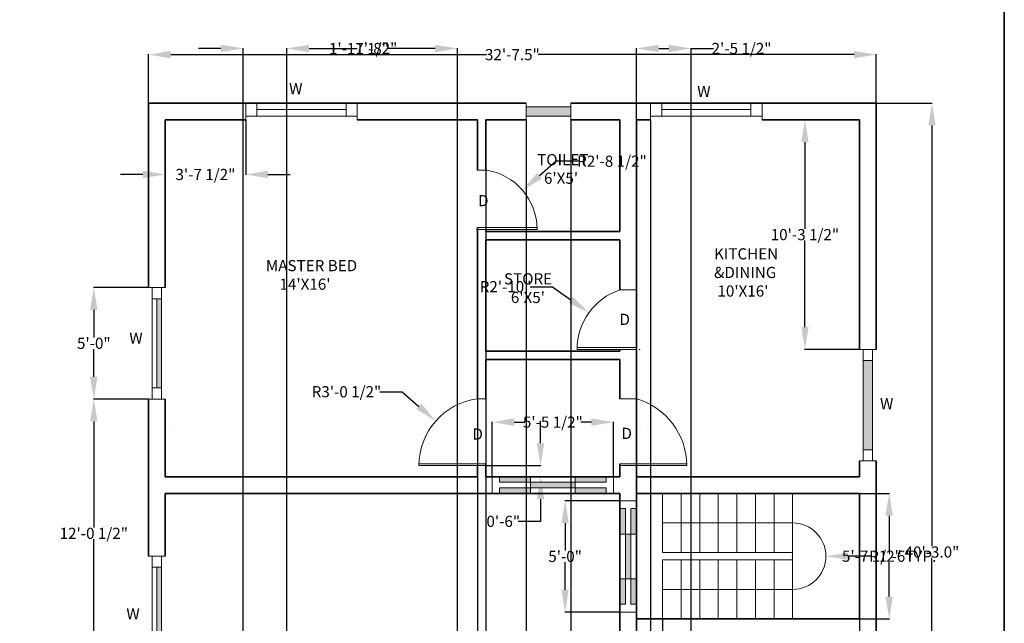
# Model space of a CAD drawing. Units: inches. Extents: x 115 to 1174, y 222 to 1302.
# Tile 4 of 5: x 644 to 1174, y 521 to 846. Entities that reach past the tile are written whole.
import ezdxf

# ---------------------------------------------------------------- set-up
doc = ezdxf.new("R2010")
doc.units = ezdxf.units.IN
doc.header["$MEASUREMENT"] = 0
for name, color, linetype, lineweight in [('A-ANNO-DIMS', 2, 'Continuous', 18), ('A-ANNO-IDEN', 7, 'Continuous', 13), ('A-ANNO-TTLB', 7, 'Continuous', 35), ('A-AREA-IDEN', 7, 'Continuous', 18), ('A-DOOR', 3, 'Continuous', 18), ('A-FLOR-STRS', 7, 'Continuous', 18), ('A-GLAZ', 4, 'Continuous', 18), ('A-GLAZ-PATT', 8, 'Continuous', 13), ('A-WALL', 7, 'Continuous', 35)]:
    doc.layers.add(name, color=color, linetype=linetype, lineweight=lineweight)
doc.styles.get("Standard").update_dxf_attribs({"font": 'arial.ttf'})
doc.dimstyles.get("Standard").update_dxf_attribs({"dimtxt": 6, "dimasz": 12, "dimexe": 0.18, "dimexo": 0.0625, "dimgap": 0.09, "dimtad": 0, "dimtih": 1, "dimtoh": 1, "dimdec": 1, "dimzin": 0, "dimdsep": 46, "dimlunit": 3, "dimtxsty": 'Standard', "dimcen": 0.09, "dimadec": 0, "dimazin": 0, "dimtfac": 1, "dimtdec": 1, "dimtofl": 0, "dimtmove": 0, "dimatfit": 3, "dimfxl": 1, "dimtolj": 1, "dimtzin": 0, "dimarcsym": 0})

# ---------------------------------------------------------------- blocks, each defined once
blk = doc.blocks.new('*D3')
at = {"layer": 'A-ANNO-DIMS', "color": 0, "lineweight": -2, "transparency": 16777216}
for p, q in [((713.72, 801.13), (713.72, 827.33)), ((725.72, 827.15), (895.58, 827.15)), ((1093.22, 827.15), (923.36, 827.15)), ((1105.22, 801.13), (1105.22, 827.33))]:
    blk.add_line(p, q, dxfattribs=at)
at = {"layer": 'A-ANNO-DIMS', "color": 0, "transparency": 16777216}
for points in [[(725.72, 829.15), (725.72, 825.15), (713.72, 827.15)], [(1093.22, 829.15), (1093.22, 825.15), (1105.22, 827.15)]]:
    blk.add_solid(points, dxfattribs=at)
at = {"layer": 'Defpoints', "color": 0, "transparency": 16777216}
for p in [(1105.22, 827.15), (713.72, 801.06), (1105.22, 801.06)]:
    blk.add_point(p, dxfattribs=at)
at = {"layer": 'A-ANNO-DIMS', "color": 0, "transparency": 16777216, "insert": (909.47, 827.15), "char_height": 6, "attachment_point": 5}
blk.add_mtext('\\A1;32\'-7.5"', dxfattribs=at)
blk = doc.blocks.new('*D4')
at = {"layer": 'A-ANNO-DIMS', "color": 0, "lineweight": -2, "transparency": 16777216}
for p, q in [((1105.28, 801.06), (1135.32, 801.06)), ((1135.14, 789.06), (1135.14, 562.72)), ((1135.14, 330.06), (1135.14, 556.41)), ((1105.28, 318.06), (1135.32, 318.06))]:
    blk.add_line(p, q, dxfattribs=at)
at = {"layer": 'A-ANNO-DIMS', "color": 0, "transparency": 16777216}
for points in [[(1133.14, 789.06), (1137.14, 789.06), (1135.14, 801.06)], [(1133.14, 330.06), (1137.14, 330.06), (1135.14, 318.06)]]:
    blk.add_solid(points, dxfattribs=at)
at = {"layer": 'Defpoints', "color": 0, "transparency": 16777216}
for p in [(1105.22, 801.06), (1105.22, 318.06), (1135.14, 318.06)]:
    blk.add_point(p, dxfattribs=at)
at = {"layer": 'A-ANNO-DIMS', "color": 0, "transparency": 16777216, "insert": (1135.14, 559.56), "char_height": 6, "attachment_point": 5}
blk.add_mtext('\\A1;40\'-3.0"', dxfattribs=at)
blk = doc.blocks.new('DOOR-36-SWING')
for p, q in [((0, 0), (0, 36)), ((0, 36), (0, 0)), ((1, 36), (1, 0)), ((36, 0), (36, 9)), ((0, 0), (1, 0))]:
    blk.add_line(p, q)
blk.add_arc((0, -1.5), 37.5, 16.2602, 90)
blk = doc.blocks.new('DOOR-32-SWING')
for p, q in [((32, 32), (23, 32)), ((0, 1), (32, 1)), ((32, 0), (0, 0)), ((0, 0), (32, 0)), ((32, 0), (32, 1))]:
    blk.add_line(p, q)
blk.add_arc((33.76, 0), 33.76, 108.5866, 180)
blk = doc.blocks.new('DOOR-32-PARTITION')
for p, q in [((0, 32), (4.5, 32)), ((0, 0), (0, 1)), ((32, 1), (0, 1)), ((0, 0), (32, 0)), ((32, 0), (0, 0))]:
    blk.add_line(p, q)
blk.add_arc((-0.37, 0), 32.37, 0, 81.3499)
blk = doc.blocks.new('STAIR-HALF-TURN')
for p, q in [((0, 67.5), (0, 35.75)), ((10, 67.5), (10, 35.75)), ((20, 67.5), (20, 35.75)), ((30, 67.5), (30, 35.75)), ((40, 67.5), (40, 35.75)), ((50, 67.5), (50, 35.75)), ((60, 67.5), (60, 35.75)), ((70, 67.5), (70, 0)), ((106, 67.5), (106, 0)), ((0, 51.63), (70, 51.63)), ((70, 35.75), (0, 35.75)), ((70, 31.75), (0, 31.75)), ((0, 31.75), (0, 0)), ((10, 31.75), (10, 0)), ((20, 31.75), (20, 0)), ((30, 31.75), (30, 0)), ((40, 31.75), (40, 0)), ((50, 31.75), (50, 0)), ((60, 31.75), (60, 0)), ((0, 15.88), (70, 15.88))]:
    blk.add_line(p, q)
blk.add_arc((70, 33.75), 17.88, 270, 90)
blk = doc.blocks.new('WIN-60-RECESSED')
for p, q in [((0, 9), (0, 0)), ((60, 9), (0, 9)), ((6, 9), (6, 2)), ((6, 5.5), (54, 5.5)), ((54, 2), (54, 9)), ((60, 0), (60, 9)), ((0, 2), (60, 2))]:
    blk.add_line(p, q)
blk = doc.blocks.new('*D27')
at = {"layer": 'A-ANNO-DIMS', "color": 0, "lineweight": -2, "transparency": 16777216}
for p, q in [((990.22, 523.5), (990.22, 507.48)), ((1096.22, 523.5), (1096.22, 507.48)), ((1002.22, 507.66), (1009.02, 507.66)), ((1084.22, 507.66), (1077.42, 507.66))]:
    blk.add_line(p, q, dxfattribs=at)
at = {"layer": 'A-ANNO-DIMS', "color": 0, "transparency": 16777216}
for points in [[(1002.22, 509.66), (1002.22, 505.66), (990.22, 507.66)], [(1084.22, 509.66), (1084.22, 505.66), (1096.22, 507.66)]]:
    blk.add_solid(points, dxfattribs=at)
at = {"layer": 'Defpoints', "color": 0, "transparency": 16777216}
for p in [(990.22, 523.56), (1096.22, 523.56), (1096.22, 507.66)]:
    blk.add_point(p, dxfattribs=at)
at = {"layer": 'A-ANNO-DIMS', "color": 0, "transparency": 16777216, "insert": (1043.22, 507.66), "char_height": 6, "attachment_point": 5}
blk.add_mtext('\\A1;STAIR 8\'-10" TYP.', dxfattribs=at)
blk = doc.blocks.new('*D28')
at = {"layer": 'A-ANNO-DIMS', "color": 0, "lineweight": -2, "transparency": 16777216}
for p, q in [((1096.28, 591.06), (1112.3, 591.06)), ((1112.12, 579.06), (1112.12, 560.51)), ((1112.12, 535.56), (1112.12, 554.12)), ((1096.28, 523.56), (1112.3, 523.56))]:
    blk.add_line(p, q, dxfattribs=at)
at = {"layer": 'A-ANNO-DIMS', "color": 0, "transparency": 16777216}
for points in [[(1110.12, 579.06), (1114.12, 579.06), (1112.12, 591.06)], [(1110.12, 535.56), (1114.12, 535.56), (1112.12, 523.56)]]:
    blk.add_solid(points, dxfattribs=at)
at = {"layer": 'Defpoints', "color": 0, "transparency": 16777216}
for p in [(1096.22, 591.06), (1112.12, 591.06), (1096.22, 523.56)]:
    blk.add_point(p, dxfattribs=at)
at = {"layer": 'A-ANNO-DIMS', "color": 0, "transparency": 16777216, "insert": (1112.12, 557.31), "char_height": 6, "attachment_point": 5}
blk.add_mtext('\\A1;5\'-7 1/2" TYP.', dxfattribs=at)
blk = doc.blocks.new('*D53')
at = {"layer": 'A-ANNO-DIMS', "color": 0, "lineweight": -2, "transparency": 16777216}
for p, q in [((713.66, 641.84), (684.14, 641.84)), ((684.32, 629.84), (684.32, 572.79)), ((684.32, 509.36), (684.32, 566.41)), ((713.66, 497.36), (684.14, 497.36))]:
    blk.add_line(p, q, dxfattribs=at)
at = {"layer": 'A-ANNO-DIMS', "color": 0, "transparency": 16777216}
for points in [[(682.32, 629.84), (686.32, 629.84), (684.32, 641.84)], [(682.32, 509.36), (686.32, 509.36), (684.32, 497.36)]]:
    blk.add_solid(points, dxfattribs=at)
at = {"layer": 'Defpoints', "color": 0, "transparency": 16777216}
for p in [(684.32, 641.84), (713.72, 641.84), (713.72, 497.36)]:
    blk.add_point(p, dxfattribs=at)
at = {"layer": 'A-ANNO-DIMS', "color": 0, "transparency": 16777216, "insert": (684.32, 569.6), "char_height": 6, "attachment_point": 5}
blk.add_mtext('\\A1;12\'-0 1/2"', dxfattribs=at)
blk = doc.blocks.new('*D54')
at = {"layer": 'A-ANNO-DIMS', "color": 0, "lineweight": -2, "transparency": 16777216}
for p, q in [((713.66, 701.84), (684.14, 701.84)), ((684.32, 689.84), (684.32, 674.99)), ((684.32, 653.84), (684.32, 668.68)), ((713.66, 641.84), (684.14, 641.84))]:
    blk.add_line(p, q, dxfattribs=at)
at = {"layer": 'A-ANNO-DIMS', "color": 0, "transparency": 16777216}
for points in [[(682.32, 689.84), (686.32, 689.84), (684.32, 701.84)], [(682.32, 653.84), (686.32, 653.84), (684.32, 641.84)]]:
    blk.add_solid(points, dxfattribs=at)
at = {"layer": 'Defpoints', "color": 0, "transparency": 16777216}
for p in [(684.32, 701.84), (713.72, 701.84), (713.72, 641.84)]:
    blk.add_point(p, dxfattribs=at)
at = {"layer": 'A-ANNO-DIMS', "color": 0, "transparency": 16777216, "insert": (684.32, 671.84), "char_height": 6, "attachment_point": 5}
blk.add_mtext('\\A1;5\'-0"', dxfattribs=at)
blk = doc.blocks.new('*D56')
at = {"layer": 'A-ANNO-DIMS', "color": 0, "lineweight": -2, "transparency": 16777216}
for p, q in [((1096.16, 792.06), (1066.64, 792.06)), ((1066.82, 780.06), (1066.82, 733.5)), ((1066.82, 680.55), (1066.82, 727.11)), ((1096.16, 668.55), (1066.64, 668.55))]:
    blk.add_line(p, q, dxfattribs=at)
at = {"layer": 'A-ANNO-DIMS', "color": 0, "transparency": 16777216}
for points in [[(1064.82, 780.06), (1068.82, 780.06), (1066.82, 792.06)], [(1064.82, 680.55), (1068.82, 680.55), (1066.82, 668.55)]]:
    blk.add_solid(points, dxfattribs=at)
at = {"layer": 'Defpoints', "color": 0, "transparency": 16777216}
for p in [(1066.82, 792.06), (1096.22, 792.06), (1096.22, 668.55)]:
    blk.add_point(p, dxfattribs=at)
at = {"layer": 'A-ANNO-DIMS', "color": 0, "transparency": 16777216, "insert": (1066.82, 730.31), "char_height": 6, "attachment_point": 5}
blk.add_mtext('\\A1;10\'-3 1/2"', dxfattribs=at)
blk = doc.blocks.new('*D57')
at = {"layer": 'A-ANNO-DIMS', "color": 0, "lineweight": -2, "transparency": 16777216}
for p, q in [((722.722051, 792.001973), (722.722051, 762.484473)), ((766.009807, 792.001973), (766.009807, 762.484473)), ((710.722051, 762.664473), (698.722051, 762.664473)), ((778.009807, 762.664473), (790.009807, 762.664473))]:
    blk.add_line(p, q, dxfattribs=at)
at = {"layer": 'A-ANNO-DIMS', "color": 0, "transparency": 16777216}
for points in [[(710.722051, 764.664473), (710.722051, 760.664473), (722.722051, 762.664473)], [(778.009807, 764.664473), (778.009807, 760.664473), (766.009807, 762.664473)]]:
    blk.add_solid(points, dxfattribs=at)
at = {"layer": 'Defpoints', "color": 0, "transparency": 16777216}
for p in [(722.722051, 792.064473), (766.009807, 792.064473), (722.722051, 762.664473)]:
    blk.add_point(p, dxfattribs=at)
at = {"layer": 'A-ANNO-DIMS', "color": 0, "transparency": 16777216, "insert": (744.365929, 762.664473), "char_height": 6, "attachment_point": 5}
blk.add_mtext('\\A1;3\'-7 1/2"', dxfattribs=at)
blk = doc.blocks.new('*D58')
at = {"layer": 'A-ANNO-DIMS', "color": 0, "lineweight": -2, "transparency": 16777216}
for p, q in [((895.22, 792), (895.22, 242.01)), ((916.83, 792), (916.83, 242.01)), ((883.22, 242.19), (871.22, 242.19)), ((928.83, 242.19), (940.83, 242.19))]:
    blk.add_line(p, q, dxfattribs=at)
at = {"layer": 'A-ANNO-DIMS', "color": 0, "transparency": 16777216}
for points in [[(883.22, 244.19), (883.22, 240.19), (895.22, 242.19)], [(928.83, 244.19), (928.83, 240.19), (916.83, 242.19)]]:
    blk.add_solid(points, dxfattribs=at)
at = {"layer": 'Defpoints', "color": 0, "transparency": 16777216}
for p in [(895.22, 792.06), (916.83, 792.06), (916.83, 242.19)]:
    blk.add_point(p, dxfattribs=at)
at = {"layer": 'A-ANNO-DIMS', "color": 0, "transparency": 16777216, "insert": (955.6, 242.19), "char_height": 6, "attachment_point": 5}
blk.add_mtext('\\A1;1\'-9 1/2"', dxfattribs=at)
blk = doc.blocks.new('*D59')
at = {"layer": 'A-ANNO-DIMS', "color": 0, "lineweight": -2, "transparency": 16777216}
for p, q in [((916.831751, 792.001973), (916.831751, 242.009173)), ((940.831751, 792.001973), (940.831751, 242.009173)), ((904.831751, 242.189173), (892.831751, 242.189173)), ((952.831751, 242.189173), (964.831751, 242.189173))]:
    blk.add_line(p, q, dxfattribs=at)
at = {"layer": 'A-ANNO-DIMS', "color": 0, "transparency": 16777216}
for points in [[(904.831751, 244.189173), (904.831751, 240.189173), (916.831751, 242.189173)], [(952.831751, 244.189173), (952.831751, 240.189173), (940.831751, 242.189173)]]:
    blk.add_solid(points, dxfattribs=at)
at = {"layer": 'Defpoints', "color": 0, "transparency": 16777216}
for p in [(916.831751, 792.064473), (940.831751, 792.064473), (940.831751, 242.189173)]:
    blk.add_point(p, dxfattribs=at)
at = {"layer": 'A-ANNO-DIMS', "color": 0, "transparency": 16777216, "insert": (928.831751, 242.189173), "char_height": 6, "attachment_point": 5}
blk.add_mtext('\\A1;2\'-0"', dxfattribs=at)
blk = doc.blocks.new('*D60')
at = {"layer": 'A-ANNO-DIMS', "color": 0, "lineweight": -2, "transparency": 16777216}
for p, q in [((976.22, 792), (976.22, 242.01)), ((983.78, 792), (983.78, 242.01)), ((964.22, 242.19), (952.22, 242.19)), ((995.78, 242.19), (1007.78, 242.19))]:
    blk.add_line(p, q, dxfattribs=at)
at = {"layer": 'A-ANNO-DIMS', "color": 0, "transparency": 16777216}
for points in [[(964.22, 244.19), (964.22, 240.19), (976.22, 242.19)], [(995.78, 244.19), (995.78, 240.19), (983.78, 242.19)]]:
    blk.add_solid(points, dxfattribs=at)
at = {"layer": 'Defpoints', "color": 0, "transparency": 16777216}
for p in [(976.22, 792.06), (983.78, 792.06), (983.78, 242.19)]:
    blk.add_point(p, dxfattribs=at)
at = {"layer": 'A-ANNO-DIMS', "color": 0, "transparency": 16777216, "insert": (1022.83, 242.19), "char_height": 6, "attachment_point": 5}
blk.add_mtext('\\A1;0\'-7 1/2"', dxfattribs=at)
blk = doc.blocks.new('*D62')
at = {"layer": 'A-ANNO-DIMS', "color": 0, "lineweight": -2, "transparency": 16777216}
for p, q in [((752.72, 830.46), (740.72, 830.46)), ((764.72, 327.13), (764.72, 830.64)), ((788.09, 327.13), (788.09, 830.64)), ((800.09, 830.46), (812.09, 830.46))]:
    blk.add_line(p, q, dxfattribs=at)
at = {"layer": 'A-ANNO-DIMS', "color": 0, "transparency": 16777216}
for points in [[(752.72, 832.46), (752.72, 828.46), (764.72, 830.46)], [(800.09, 832.46), (800.09, 828.46), (788.09, 830.46)]]:
    blk.add_solid(points, dxfattribs=at)
at = {"layer": 'Defpoints', "color": 0, "transparency": 16777216}
for p in [(788.09, 830.46), (764.72, 327.06), (788.09, 327.06)]:
    blk.add_point(p, dxfattribs=at)
at = {"layer": 'A-ANNO-DIMS', "color": 0, "transparency": 16777216, "insert": (829.19, 830.46), "char_height": 6, "attachment_point": 5}
blk.add_mtext('\\A1;1\'-11 1/2"', dxfattribs=at)
blk = doc.blocks.new('*D63')
at = {"layer": 'A-ANNO-DIMS', "color": 0, "lineweight": -2, "transparency": 16777216}
for p, q in [((788.09, 327.13), (788.09, 830.64)), ((800.09, 830.46), (825.98, 830.46)), ((867.96, 830.46), (842.06, 830.46)), ((879.96, 327.13), (879.96, 830.64))]:
    blk.add_line(p, q, dxfattribs=at)
at = {"layer": 'A-ANNO-DIMS', "color": 0, "transparency": 16777216}
for points in [[(800.09, 832.46), (800.09, 828.46), (788.09, 830.46)], [(867.96, 832.46), (867.96, 828.46), (879.96, 830.46)]]:
    blk.add_solid(points, dxfattribs=at)
at = {"layer": 'Defpoints', "color": 0, "transparency": 16777216}
for p in [(879.96, 830.46), (788.09, 327.06), (879.96, 327.06)]:
    blk.add_point(p, dxfattribs=at)
at = {"layer": 'A-ANNO-DIMS', "color": 0, "transparency": 16777216, "insert": (834.02, 830.46), "char_height": 6, "attachment_point": 5}
blk.add_mtext('\\A1;7\'-8"', dxfattribs=at)
blk = doc.blocks.new('*D64')
at = {"layer": 'A-ANNO-DIMS', "color": 0, "lineweight": -2, "transparency": 16777216}
for p, q in [((976.22, 327.13), (976.22, 830.64)), ((988.22, 830.46), (993.61, 830.46)), ((1005.61, 327.13), (1005.61, 830.64)), ((1005.61, 830.46), (1017.61, 830.46))]:
    blk.add_line(p, q, dxfattribs=at)
at = {"layer": 'A-ANNO-DIMS', "color": 0, "transparency": 16777216}
for points in [[(988.22, 832.46), (988.22, 828.46), (976.22, 830.46)], [(993.61, 832.46), (993.61, 828.46), (1005.61, 830.46)]]:
    blk.add_solid(points, dxfattribs=at)
at = {"layer": 'Defpoints', "color": 0, "transparency": 16777216}
for p in [(1005.61, 830.46), (976.22, 327.06), (1005.61, 327.06)]:
    blk.add_point(p, dxfattribs=at)
at = {"layer": 'A-ANNO-DIMS', "color": 0, "transparency": 16777216, "insert": (1032.72, 830.46), "char_height": 6, "attachment_point": 5}
blk.add_mtext('\\A1;2\'-5 1/2"', dxfattribs=at)
blk = doc.blocks.new('*D67')
at = {"layer": 'A-ANNO-DIMS', "color": 0, "lineweight": -2, "transparency": 16777216}
for p, q in [((890.72, 733), (890.72, 242.01)), ((895.22, 727.5), (895.22, 242.01)), ((878.72, 242.19), (866.72, 242.19)), ((907.22, 242.19), (919.22, 242.19))]:
    blk.add_line(p, q, dxfattribs=at)
at = {"layer": 'A-ANNO-DIMS', "color": 0, "transparency": 16777216}
for points in [[(878.72, 244.19), (878.72, 240.19), (890.72, 242.19)], [(907.22, 244.19), (907.22, 240.19), (895.22, 242.19)]]:
    blk.add_solid(points, dxfattribs=at)
at = {"layer": 'Defpoints', "color": 0, "transparency": 16777216}
for p in [(890.72, 733.06), (895.22, 727.56), (895.22, 242.19)]:
    blk.add_point(p, dxfattribs=at)
at = {"layer": 'A-ANNO-DIMS', "color": 0, "transparency": 16777216, "insert": (934.28, 242.19), "char_height": 6, "attachment_point": 5}
blk.add_mtext('\\A1;0\'-4 1/2"', dxfattribs=at)
blk = doc.blocks.new('*D68')
at = {"layer": 'A-ANNO-DIMS', "color": 0, "lineweight": -2, "transparency": 16777216}
for p, q in [((898.51, 600.13), (898.51, 629.64)), ((910.51, 629.46), (916.17, 629.46)), ((951.94, 629.46), (946.28, 629.46)), ((963.94, 600.13), (963.94, 629.64))]:
    blk.add_line(p, q, dxfattribs=at)
at = {"layer": 'A-ANNO-DIMS', "color": 0, "transparency": 16777216}
for points in [[(910.51, 631.46), (910.51, 627.46), (898.51, 629.46)], [(951.94, 631.46), (951.94, 627.46), (963.94, 629.46)]]:
    blk.add_solid(points, dxfattribs=at)
at = {"layer": 'Defpoints', "color": 0, "transparency": 16777216}
for p in [(963.94, 629.46), (898.51, 600.06), (963.94, 600.06)]:
    blk.add_point(p, dxfattribs=at)
at = {"layer": 'A-ANNO-DIMS', "color": 0, "transparency": 16777216, "insert": (931.23, 629.46), "char_height": 6, "attachment_point": 5}
blk.add_mtext('\\A1;5\'-5 1/2"', dxfattribs=at)
blk = doc.blocks.new('*D69')
at = {"layer": 'A-ANNO-DIMS', "color": 0, "lineweight": -2, "transparency": 16777216}
for p, q in [((967.16, 587.16), (937.64, 587.16)), ((937.82, 575.16), (937.82, 560.38)), ((937.82, 539.29), (937.82, 554.07)), ((967.16, 527.29), (937.64, 527.29))]:
    blk.add_line(p, q, dxfattribs=at)
at = {"layer": 'A-ANNO-DIMS', "color": 0, "transparency": 16777216}
for points in [[(935.82, 575.16), (939.82, 575.16), (937.82, 587.16)], [(935.82, 539.29), (939.82, 539.29), (937.82, 527.29)]]:
    blk.add_solid(points, dxfattribs=at)
at = {"layer": 'Defpoints', "color": 0, "transparency": 16777216}
for p in [(937.82, 587.16), (967.22, 587.16), (967.22, 527.29)]:
    blk.add_point(p, dxfattribs=at)
at = {"layer": 'A-ANNO-DIMS', "color": 0, "transparency": 16777216, "insert": (937.82, 557.22), "char_height": 6, "attachment_point": 5}
blk.add_mtext('\\A1;5\'-0"', dxfattribs=at)
blk = doc.blocks.new('*D70')
at = {"layer": 'A-ANNO-DIMS', "color": 0, "lineweight": -2, "transparency": 16777216}
for p, q in [((924.62, 618.06), (924.62, 630.06)), ((895.28, 606.06), (924.8, 606.06)), ((895.28, 600.06), (924.8, 600.06)), ((924.62, 588.06), (924.62, 576.06)), ((924.62, 576.06), (912.62, 576.06))]:
    blk.add_line(p, q, dxfattribs=at)
at = {"layer": 'A-ANNO-DIMS', "color": 0, "transparency": 16777216}
for points in [[(922.62, 618.06), (926.62, 618.06), (924.62, 606.06)], [(922.62, 588.06), (926.62, 588.06), (924.62, 600.06)]]:
    blk.add_solid(points, dxfattribs=at)
at = {"layer": 'Defpoints', "color": 0, "transparency": 16777216}
for p in [(895.22, 606.06), (895.22, 600.06), (924.62, 600.06)]:
    blk.add_point(p, dxfattribs=at)
at = {"layer": 'A-ANNO-DIMS', "color": 0, "transparency": 16777216, "insert": (904.56, 576.06), "char_height": 6, "attachment_point": 5}
blk.add_mtext('\\A1;0\'-6"', dxfattribs=at)
blk = doc.blocks.new('*D93')
at = {"layer": 'A-ANNO-DIMS', "color": 0, "lineweight": -2, "transparency": 16777216}
for p, q in [((838.15, 645.79), (850.15, 645.79)), ((850.15, 645.79), (859.18, 637.88)), ((895.45, 606.06), (895.63, 606.06)), ((895.54, 605.97), (895.54, 606.15))]:
    blk.add_line(p, q, dxfattribs=at)
at = {"layer": 'A-ANNO-DIMS', "color": 0, "transparency": 16777216}
blk.add_solid([(860.49, 639.39), (857.86, 636.38), (868.21, 629.98)], dxfattribs=at)
at = {"layer": 'Defpoints', "color": 0, "transparency": 16777216}
for p in [(868.21, 629.98), (895.54, 606.06)]:
    blk.add_point(p, dxfattribs=at)
at = {"layer": 'A-ANNO-DIMS', "color": 0, "transparency": 16777216, "insert": (820.22, 645.79), "char_height": 6, "attachment_point": 5}
blk.add_mtext('\\A1;R3\'-0 1/2"', dxfattribs=at)
blk = doc.blocks.new('*D95')
at = {"layer": 'A-ANNO-DIMS', "color": 0, "lineweight": -2, "transparency": 16777216}
for p, q in [((919.08, 702.28), (931.08, 702.28)), ((931.08, 702.28), (940.82, 695.27)), ((977.89, 668.56), (978.07, 668.56)), ((977.98, 668.47), (977.98, 668.65))]:
    blk.add_line(p, q, dxfattribs=at)
at = {"layer": 'A-ANNO-DIMS', "color": 0, "transparency": 16777216}
blk.add_solid([(941.99, 696.9), (939.66, 693.65), (950.57, 688.27)], dxfattribs=at)
at = {"layer": 'Defpoints', "color": 0, "transparency": 16777216}
for p in [(950.57, 688.27), (977.98, 668.56)]:
    blk.add_point(p, dxfattribs=at)
at = {"layer": 'A-ANNO-DIMS', "color": 0, "transparency": 16777216, "insert": (905.81, 702.28), "char_height": 6, "attachment_point": 5}
blk.add_mtext('\\A1;R2\'-10"', dxfattribs=at)
blk = doc.blocks.new('*D96')
at = {"layer": 'A-ANNO-DIMS', "color": 0, "lineweight": -2, "transparency": 16777216}
for p, q in [((933.1, 769.8), (924, 761.98)), ((945.1, 769.8), (933.1, 769.8)), ((890.26, 733.06), (890.44, 733.06)), ((890.35, 732.97), (890.35, 733.15))]:
    blk.add_line(p, q, dxfattribs=at)
at = {"layer": 'A-ANNO-DIMS', "color": 0, "transparency": 16777216}
blk.add_solid([(922.7, 763.5), (925.31, 760.47), (914.9, 754.16)], dxfattribs=at)
at = {"layer": 'Defpoints', "color": 0, "transparency": 16777216}
for p in [(914.9, 754.16), (890.35, 733.06)]:
    blk.add_point(p, dxfattribs=at)
at = {"layer": 'A-ANNO-DIMS', "color": 0, "transparency": 16777216, "insert": (963.03, 769.8), "char_height": 6, "attachment_point": 5}
blk.add_mtext('\\A1;R2\'-8 1/2"', dxfattribs=at)
blk = doc.blocks.new('*D97')
at = {"layer": 'A-ANNO-DIMS', "color": 0, "lineweight": -2, "transparency": 16777216}
for p, q in [((1060.13, 557.31), (1060.31, 557.31)), ((1060.22, 557.22), (1060.22, 557.4)), ((1102.1, 557.31), (1090.1, 557.31))]:
    blk.add_line(p, q, dxfattribs=at)
at = {"layer": 'A-ANNO-DIMS', "color": 0, "transparency": 16777216}
blk.add_solid([(1090.1, 559.31), (1090.1, 555.31), (1078.1, 557.31)], dxfattribs=at)
at = {"layer": 'Defpoints', "color": 0, "transparency": 16777216}
for p in [(1060.22, 557.31), (1078.1, 557.31)]:
    blk.add_point(p, dxfattribs=at)
at = {"layer": 'A-ANNO-DIMS', "color": 0, "transparency": 16777216, "insert": (1113.03, 557.31), "char_height": 6, "attachment_point": 5}
blk.add_mtext('\\A1;R1\'-6"', dxfattribs=at)

msp = doc.modelspace()

# ---------------------------------------------------------------- hatches: boundary and pattern name
at = {"layer": 'A-GLAZ-PATT'}
h = msp.add_hatch(color=256, dxfattribs=at)
h.dxf.hatch_style = 1
h.paths.add_polyline_path([(940.83, 799.06), (916.83, 799.06), (916.83, 794.06), (940.83, 794.06)])
h = msp.add_hatch(color=256, dxfattribs=at)
h.dxf.hatch_style = 1
h.paths.add_polyline_path([(720.72, 695.84), (718.22, 695.84), (718.22, 647.84), (720.72, 647.84)])
h.paths.add_polyline_path([(720.72, 551.36), (718.22, 551.36), (718.22, 503.36), (720.72, 503.36)])
h.paths.add_polyline_path([(720.72, 444.28), (718.22, 444.28), (718.22, 396.28), (720.72, 396.28)])
h = msp.add_hatch(color=256, dxfattribs=at)
h.dxf.hatch_style = 1
h.paths.add_polyline_path([(1103.22, 662.55), (1098.22, 662.55), (1098.22, 614.55), (1103.22, 614.55)])
h.paths.add_polyline_path([(1103.22, 435.27), (1098.22, 435.27), (1098.22, 387.27), (1103.22, 387.27)])
h = msp.add_hatch(color=256, dxfattribs=at)
h.dxf.hatch_style = 1
h.paths.add_polyline_path([(919.22, 600.06), (902.51, 600.06), (902.51, 597.06), (919.22, 597.06)])
h.paths.add_polyline_path([(919.22, 594.06), (902.51, 594.06), (902.51, 591.06), (919.22, 591.06)])
h.paths.add_polyline_path([(943.22, 597.06), (919.22, 597.06), (919.22, 594.06), (943.22, 594.06)])
h.paths.add_polyline_path([(959.94, 600.06), (943.22, 600.06), (943.22, 597.06), (959.94, 597.06)])
h.paths.add_polyline_path([(959.94, 594.06), (943.22, 594.06), (943.22, 591.06), (959.94, 591.06)])
h = msp.add_hatch(color=256, dxfattribs=at)
h.dxf.hatch_style = 1
h.paths.add_polyline_path([(976.22, 582.97), (973.22, 582.97), (973.22, 569.22), (976.22, 569.22)])
h.paths.add_polyline_path([(970.22, 582.97), (967.22, 582.97), (967.22, 569.22), (970.22, 569.22)])
h.paths.add_polyline_path([(973.22, 569.22), (970.22, 569.22), (970.22, 545.22), (973.22, 545.22)])
h.paths.add_polyline_path([(976.22, 545.22), (973.22, 545.22), (973.22, 531.52), (976.22, 531.52)])
h.paths.add_polyline_path([(970.22, 545.22), (967.22, 545.22), (967.22, 531.52), (970.22, 531.52)])

# ---------------------------------------------------------------- linework, layer by layer
at = {"layer": 'A-ANNO-TTLB'}
msp.add_lwpolyline([(114.85, 1302.15), (1174.06, 1302.15), (1174.06, 222.13), (114.85, 222.13)], close=True, dxfattribs=at)
at = {"layer": 'A-DOOR'}
for p, q in [((895.22, 642.06), (890.72, 642.06)), ((726.72, 627.06), (726.72, 627.05)), ((978.22, 627.06), (978.22, 627.05)), ((859.22, 607.06), (895.22, 607.06)), ((895.22, 606.06), (859.22, 606.06)), ((859.22, 606.06), (895.22, 606.06)), ((895.22, 606.06), (895.22, 607.06))]:
    msp.add_line(p, q, dxfattribs=at)
msp.add_arc((895.54, 606.06), 36.32, 97.6281, 180, dxfattribs=at)
at = {"layer": 'A-GLAZ'}
for p, q in [((916.83, 801.06), (916.83, 792.06)), ((940.83, 792.06), (940.83, 801.06)), ((940.83, 799.06), (916.83, 799.06)), ((916.83, 794.06), (940.83, 794.06)), ((713.72, 701.84), (722.72, 701.84)), ((715.72, 641.84), (715.72, 701.84)), ((720.72, 701.84), (720.72, 641.84)), ((715.72, 695.84), (720.72, 695.84)), ((718.22, 695.84), (718.22, 647.84)), ((1096.22, 668.55), (1105.22, 668.55)), ((1098.22, 608.55), (1098.22, 668.55)), ((1103.22, 668.55), (1103.22, 608.55)), ((1098.22, 662.55), (1103.22, 662.55)), ((720.72, 647.84), (715.72, 647.84)), ((722.72, 641.84), (713.72, 641.84)), ((1103.22, 614.55), (1098.22, 614.55)), ((1105.22, 608.55), (1096.22, 608.55)), ((898.51, 600.06), (898.51, 591.06)), ((902.51, 600.06), (902.51, 597.06)), ((919.22, 600.06), (902.51, 600.06)), ((919.22, 600.06), (919.22, 591.06)), ((959.94, 600.06), (943.22, 600.06)), ((943.22, 600.06), (943.22, 591.06)), ((959.94, 597.06), (959.94, 600.06)), ((963.94, 591.06), (963.94, 600.06)), ((959.94, 597.06), (902.51, 597.06)), ((902.51, 594.06), (959.94, 594.06)), ((902.51, 594.06), (902.51, 591.06)), ((959.94, 591.06), (959.94, 594.06)), ((902.51, 591.06), (919.22, 591.06)), ((943.22, 591.06), (959.94, 591.06)), ((976.22, 587.16), (967.22, 587.16)), ((967.22, 587.16), (967.22, 527.29)), ((967.22, 582.97), (970.22, 582.97)), ((970.22, 582.97), (970.22, 531.52)), ((973.22, 531.52), (973.22, 582.97)), ((973.22, 582.97), (976.22, 582.97)), ((976.22, 527.29), (976.22, 587.16)), ((976.22, 569.22), (967.22, 569.22)), ((713.72, 557.36), (722.72, 557.36)), ((715.72, 497.36), (715.72, 557.36)), ((720.72, 557.36), (720.72, 497.36)), ((715.72, 551.36), (720.72, 551.36)), ((718.22, 551.36), (718.22, 503.36)), ((976.22, 545.22), (967.22, 545.22)), ((967.22, 527.29), (967.22, 531.52)), ((967.22, 531.52), (970.22, 531.52)), ((973.22, 531.52), (976.22, 531.52)), ((976.22, 531.52), (976.22, 527.29)), ((967.22, 527.29), (976.22, 527.29))]:
    msp.add_line(p, q, dxfattribs=at)
at = {"layer": 'A-WALL'}
for p, q in [((713.72, 801.06), (916.83, 801.06)), ((713.72, 801.06), (713.72, 701.84)), ((940.83, 801.06), (1105.22, 801.06)), ((1105.22, 801.06), (1105.22, 668.55)), ((722.72, 792.06), (766.01, 792.06)), ((722.72, 792.06), (722.72, 701.84)), ((826.01, 792.06), (890.72, 792.06)), ((890.72, 792.06), (890.72, 765.06)), ((895.22, 792.06), (916.83, 792.06)), ((895.22, 792.06), (895.22, 765.06)), ((940.83, 792.06), (967.22, 792.06)), ((967.22, 792.06), (967.22, 732.06)), ((976.22, 792.06), (983.78, 792.06)), ((976.22, 792.06), (976.22, 700.56)), ((1043.78, 792.06), (1096.22, 792.06)), ((1096.22, 792.06), (1096.22, 668.55)), ((890.72, 734.06), (890.72, 642.06)), ((890.72, 732.06), (890.72, 733.06)), ((895.22, 733.06), (895.22, 732.06)), ((895.22, 732.06), (967.22, 732.06)), ((895.22, 727.56), (967.22, 727.56)), ((895.22, 727.56), (895.22, 667.56)), ((967.22, 727.56), (967.22, 700.56)), ((895.22, 667.56), (967.22, 667.56)), ((967.22, 668.56), (967.22, 667.56)), ((976.22, 669.56), (976.22, 642.06)), ((976.22, 667.56), (976.22, 668.56)), ((895.22, 663.06), (967.22, 663.06)), ((895.22, 663.06), (895.22, 642.06)), ((967.22, 663.06), (967.22, 642.06)), ((713.72, 641.84), (713.72, 557.36)), ((722.72, 641.84), (722.72, 600.06)), ((890.72, 606.06), (890.72, 600.06)), ((895.22, 607.06), (895.22, 600.06)), ((895.22, 600.06), (895.22, 606.06)), ((967.22, 607.06), (967.22, 600.06)), ((967.22, 600.06), (967.22, 606.06)), ((976.22, 606.06), (976.22, 600.06)), ((1096.22, 608.55), (1096.22, 600.06)), ((1105.22, 608.55), (1105.22, 441.27)), ((722.72, 600.06), (725.72, 600.06)), ((722.72, 600.06), (890.72, 600.06)), ((895.22, 600.06), (896.22, 600.06)), ((895.22, 600.06), (967.22, 600.06)), ((976.22, 600.06), (977.22, 600.06)), ((976.22, 600.06), (1096.22, 600.06)), ((722.72, 591.06), (726.72, 591.06)), ((722.72, 591.06), (898.51, 591.06)), ((722.72, 591.06), (722.72, 557.36)), ((898.51, 591.06), (967.22, 591.06)), ((967.22, 591.06), (967.22, 512.06)), ((976.22, 591.06), (978.22, 591.06)), ((976.22, 591.06), (976.22, 523.56)), ((976.22, 591.06), (977.22, 591.06)), ((976.22, 591.06), (990.22, 591.06)), ((990.22, 591.06), (1096.22, 591.06)), ((1096.22, 591.06), (1096.22, 523.56)), ((976.22, 523.56), (1096.22, 523.56))]:
    msp.add_line(p, q, dxfattribs=at)

# ---------------------------------------------------------------- block references
at = {"layer": 'A-DOOR'}
for name, p in [('DOOR-32-PARTITION', (890.72, 733.06)), ('DOOR-32-SWING', (944.22, 668.56))]:
    msp.add_blockref(name, p, dxfattribs=at)
at = {"layer": 'A-DOOR', "extrusion": (0, 0, -1), "zscale": -1, "rotation": 90.00000000000018}
msp.add_blockref('DOOR-36-SWING', (-967.22, 606.06), dxfattribs=at)
at = {"layer": 'A-FLOR-STRS'}
msp.add_blockref('STAIR-HALF-TURN', (990.22, 523.56), dxfattribs=at)
at = {"layer": 'A-GLAZ'}
for p in [(766.01, 792.06), (983.78, 792.06)]:
    msp.add_blockref('WIN-60-RECESSED', p, dxfattribs=at)

# ---------------------------------------------------------------- texts
at = {"layer": 'A-ANNO-IDEN', "char_height": 6, "attachment_point": 1}
for s, width, heights, insert in [('W', 10.5593, [0], (789.38, 811.79)), ('W', 10.5593, [0], (1008.86, 810.35)), ('D', 9.3758, [0], (890.98, 751.6)), ('D', 9.3758, [0], (967.08, 687.72)), ('W', 9.7663, [6], (703.42, 677.59)), ('W', 10.5593, [0], (1107.21, 642.36)), ('D', 9.3758, [0], (887.98, 626.02)), ('D', 9.3758, [0], (968.14, 626.39)), ('W', 10.5593, [0], (701.82, 529.36))]:
    msp.add_mtext_dynamic_manual_height_columns(s, width=width, gutter_width=30, heights=heights, dxfattribs=dict(at, insert=insert))
at = {"layer": 'A-AREA-IDEN', "char_height": 6, "attachment_point": 1}
for s, width, insert in [("TOILET\\P  6'X5'", 41.5684, (922.8, 773.64)), ("KITCHEN\\P&DINING\\P 10'X16'", 70.6782, (1017.94, 722.97)), ("MASTER BED\\P    14'X16'", 61.0364, (776.88, 716.64)), ("STORE\\P  6'X5'", 36.104, (904.98, 709.52))]:
    msp.add_mtext_dynamic_manual_height_columns(s, width=width, gutter_width=30, heights=[0], dxfattribs=dict(at, insert=insert))

# ---------------------------------------------------------------- dimensions: what is measured, and where the dimension line sits
at = {"layer": 'A-ANNO-DIMS'}
for base, p1, p2, override, picture, middle in [((788.09, 830.46), (764.72, 327.06), (788.09, 327.06), {"dimdec": 1, "dimlfac": 1, "dimrnd": 0, "dimzin": 1, "dimdsep": 46, "dimlunit": 4, "dimfrac": 2}, '*D62', (829.19, 830.46)), ((1005.61, 830.46), (976.22, 327.06), (1005.61, 327.06), {"dimdec": 1, "dimlfac": 1, "dimrnd": 0, "dimzin": 1, "dimdsep": 46, "dimlunit": 4, "dimfrac": 2}, '*D64', (1032.72, 830.46)), ((879.96, 830.46), (788.09, 327.06), (879.96, 327.06), {"dimdec": 1, "dimlfac": 1, "dimrnd": 0, "dimzin": 1, "dimdsep": 46, "dimlunit": 4, "dimfrac": 2}, '*D63', (834.02, 830.46)), ((1105.22, 827.15), (713.72, 801.06), (1105.22, 801.06), {"dimclrd": 0, "dimclre": 0, "dimclrt": 0}, '*D3', (909.47, 827.15)), ((916.83, 242.19), (895.22, 792.06), (916.83, 792.06), {"dimdec": 1, "dimlfac": 1, "dimrnd": 0, "dimzin": 1, "dimdsep": 46, "dimlunit": 4, "dimfrac": 2}, '*D58', (955.6, 242.19)), ((940.83, 242.19), (916.83, 792.06), (940.83, 792.06), {"dimdec": 1, "dimlfac": 1, "dimrnd": 0, "dimzin": 1, "dimdsep": 46, "dimlunit": 4, "dimfrac": 2}, '*D59', (928.83, 242.19)), ((983.78, 242.19), (976.22, 792.06), (983.78, 792.06), {"dimdec": 1, "dimlfac": 1, "dimrnd": 0, "dimzin": 1, "dimdsep": 46, "dimlunit": 4, "dimfrac": 2}, '*D60', (1022.83, 242.19)), ((895.22, 242.19), (890.72, 733.06), (895.22, 727.56), {"dimdec": 1, "dimlfac": 1, "dimrnd": 0, "dimzin": 1, "dimdsep": 46, "dimlunit": 4, "dimfrac": 2}, '*D67', (934.28, 242.19))]:
    dim = msp.add_linear_dim(base=base, p1=p1, p2=p2, dimstyle='Standard', override=override, dxfattribs=at)
    dim.commit()
    dim.dimension.update_dxf_attribs({"geometry": picture, "text_midpoint": middle})
for base, p1, p2, angle, override, picture, middle in [((1135.14, 318.06), (1105.22, 801.06), (1105.22, 318.06), 90, {"dimclrd": 0, "dimclre": 0, "dimclrt": 0}, '*D4', (1135.14, 559.56)), ((722.72, 762.66), (766.01, 792.06), (722.72, 792.06), 180, {"dimdec": 1, "dimlfac": 1, "dimrnd": 0, "dimzin": 1, "dimdsep": 46, "dimlunit": 4, "dimfrac": 2}, '*D57', (744.37, 762.66)), ((1066.82, 792.06), (1096.22, 668.55), (1096.22, 792.06), 90, {"dimdec": 1, "dimlfac": 1, "dimrnd": 0, "dimzin": 1, "dimdsep": 46, "dimlunit": 4, "dimfrac": 2}, '*D56', (1066.82, 730.31)), ((684.32, 701.84), (713.72, 641.84), (713.72, 701.84), 90, {"dimdec": 1, "dimlfac": 1, "dimrnd": 0, "dimzin": 1, "dimdsep": 46, "dimlunit": 4, "dimfrac": 2}, '*D54', (684.32, 671.84)), ((684.32, 641.84), (713.72, 497.36), (713.72, 641.84), 90, {"dimdec": 1, "dimlfac": 1, "dimrnd": 0, "dimzin": 1, "dimdsep": 46, "dimlunit": 4, "dimfrac": 2}, '*D53', (684.32, 569.6)), ((963.94, 629.46), (898.51, 600.06), (963.94, 600.06), 0, {"dimdec": 1, "dimlfac": 1, "dimrnd": 0, "dimzin": 1, "dimdsep": 46, "dimlunit": 4, "dimfrac": 2}, '*D68', (931.23, 629.46)), ((924.62, 600.06), (895.22, 606.06), (895.22, 600.06), 270, {"dimdec": 1, "dimlfac": 1, "dimrnd": 0, "dimzin": 1, "dimdsep": 46, "dimlunit": 4, "dimfrac": 2}, '*D70', (904.56, 576.06)), ((937.82, 587.16), (967.22, 527.29), (967.22, 587.16), 90, {"dimdec": 1, "dimlfac": 1, "dimrnd": 0, "dimzin": 1, "dimdsep": 46, "dimlunit": 4, "dimfrac": 2}, '*D69', (937.82, 557.22))]:
    dim = msp.add_linear_dim(base=base, p1=p1, p2=p2, angle=angle, dimstyle='Standard', override=override, dxfattribs=at)
    dim.commit()
    dim.dimension.update_dxf_attribs({"geometry": picture, "text_midpoint": middle})
for center, mpoint, picture, middle in [((890.35, 733.06), (914.9, 754.16), '*D96', (963.03, 769.8)), ((977.98, 668.56), (950.57, 688.27), '*D95', (905.81, 702.28)), ((895.54, 606.06), (868.21, 629.98), '*D93', (820.22, 645.79)), ((1060.22, 557.31), (1078.1, 557.31), '*D97', (1113.03, 557.31))]:
    dim = msp.add_radius_dim(center=center, mpoint=mpoint, dimstyle='Standard', override={"dimdec": 1, "dimlfac": 1, "dimrnd": 0, "dimzin": 1, "dimdsep": 46, "dimlunit": 4, "dimfrac": 2}, dxfattribs=at)
    dim.commit()
    dim.dimension.update_dxf_attribs({"geometry": picture, "text_midpoint": middle})
dim = msp.add_linear_dim(base=(1112.12, 591.06), p1=(1096.22, 523.56), p2=(1096.22, 591.06), angle=90, text='<> TYP.', dimstyle='Standard', override={"dimdec": 1, "dimlfac": 1, "dimrnd": 0, "dimzin": 1, "dimdsep": 46, "dimlunit": 4, "dimfrac": 2}, dxfattribs=at)
dim.commit()
dim.dimension.update_dxf_attribs({"geometry": '*D28', "text_midpoint": (1112.12, 557.31)})
dim = msp.add_linear_dim(base=(1096.22, 507.66), p1=(990.22, 523.56), p2=(1096.22, 523.56), text='STAIR <> TYP.', dimstyle='Standard', override={"dimdec": 1, "dimlfac": 1, "dimrnd": 0, "dimzin": 1, "dimdsep": 46, "dimlunit": 4, "dimfrac": 2}, dxfattribs=at)
dim.commit()
dim.dimension.update_dxf_attribs({"geometry": '*D27', "text_midpoint": (1043.22, 507.66)})

doc.saveas('drawing.dxf')
